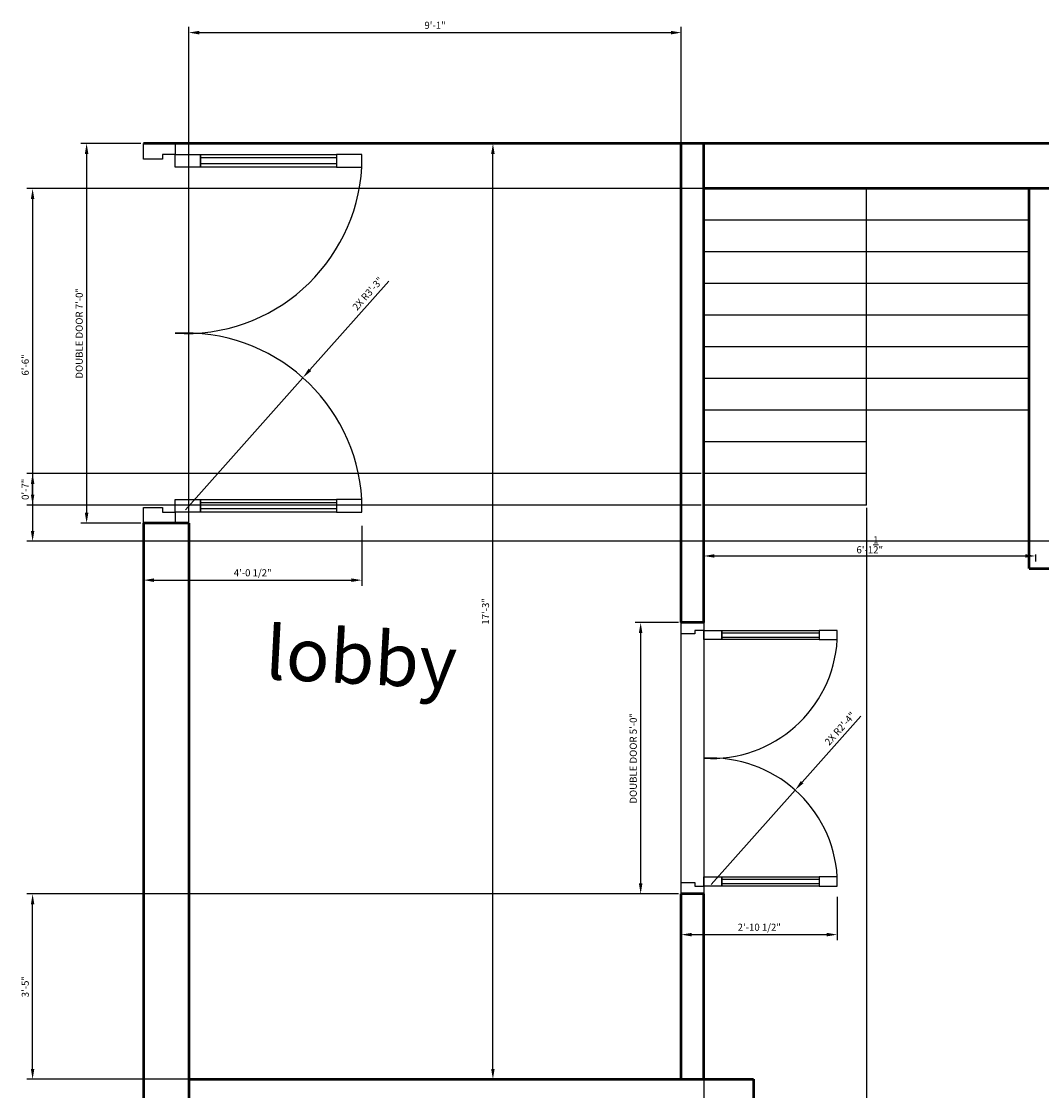
# Model space of a CAD drawing. Units: inches. Extents: x -28 to 484, y -33 to 391.
# Tile 2 of 4: x -27 to 199, y 133 to 369. Entities that reach past the tile are written whole.
import ezdxf

# ---------------------------------------------------------------- set-up
doc = ezdxf.new("R2010")
doc.units = ezdxf.units.IN
for name, color, linetype, lineweight in [('A-ANNO-DIMS', 2, 'Continuous', 18), ('A-AREA-IDEN', 7, 'Continuous', 25), ('A-DOOR', 3, 'Continuous', 25), ('A-FLOR-STRS', 7, 'Continuous', 25), ('A-WALL', 7, 'Continuous', 50)]:
    doc.layers.add(name, color=color, linetype=linetype, lineweight=lineweight)
doc.styles.get("Standard").update_dxf_attribs({"font": 'arial.ttf'})
doc.dimstyles.new('ISO-25', dxfattribs={"dimtxt": 1.5625, "dimasz": 2.3125, "dimexe": 1.25, "dimexo": 0.625, "dimtad": 1, "dimlunit": 4, "dimtxsty": 'Standard', "dimcen": 2.5, "dimadec": 0, "dimazin": 0, "dimtfac": 1, "dimtmove": 0, "dimatfit": 3, "dimfxl": 1, "dimarcsym": 0})

# ---------------------------------------------------------------- blocks, each defined once
blk = doc.blocks.new('A$C09A905BE')
for p, q in [((35, 690), (35, 610)), ((75, 690), (35, 690)), ((75, 610), (75, 690)), ((1125, 690), (1125, 610)), ((1165, 690), (1125, 690)), ((1165, 610), (1165, 690)), ((35, 610), (75, 610)), ((35, 180), (35, 610)), ((35, 610), (75, 610)), ((45, 180), (45, 610)), ((45, 610), (65, 610)), ((65, 610), (65, 180)), ((75, 610), (75, 180)), ((1125, 610), (1165, 610)), ((1125, 180), (1125, 610)), ((1125, 610), (1165, 610)), ((1135, 180), (1135, 610)), ((1135, 610), (1155, 610)), ((1155, 610), (1155, 180)), ((1165, 610), (1165, 180)), ((35, 100), (35, 180)), ((35, 180), (75, 180)), ((75, 180), (35, 180)), ((65, 180), (45, 180)), ((75, 180), (75, 100)), ((1125, 100), (1125, 180)), ((1125, 180), (1165, 180)), ((1165, 180), (1125, 180)), ((1155, 180), (1135, 180)), ((1165, 180), (1165, 100)), ((0, 0), (0, 100)), ((0, 100), (35, 100)), ((35, 100), (35, 60)), ((75, 100), (35, 100)), ((1165, 100), (1125, 100)), ((1165, 100), (1200, 100)), ((1165, 60), (1165, 100)), ((1200, 100), (1200, 0)), ((35, 60), (50, 60)), ((50, 60), (50, 50)), ((50, 50), (50, 0)), ((1150, 50), (1150, 60)), ((1150, 60), (1165, 60)), ((1150, 0), (1150, 50)), ((50, 0), (0, 0)), ((1200, 0), (1150, 0))]:
    blk.add_line(p, q)
for centre, start, end in [((42.5, 132.5), 356.6637, 86.6637), ((1157.5, 132.5), 93.3363, 183.3363)]:
    blk.add_arc(centre, 558.4, start, end)
blk = doc.blocks.new('*D13')
at = {"layer": 'A-ANNO-DIMS', "color": 0, "lineweight": -2, "transparency": 16777216}
for p, q in [((73.12, 342), (78.56, 342)), ((77.31, 137.31), (77.31, 339.69)), ((73.12, 135), (78.56, 135))]:
    blk.add_line(p, q, dxfattribs=at)
at = {"layer": 'A-ANNO-DIMS', "color": 0, "transparency": 16777216}
for points in [[(76.92, 339.69), (77.69, 339.69), (77.31, 342)], [(76.92, 137.31), (77.69, 137.31), (77.31, 135)]]:
    blk.add_solid(points, dxfattribs=at)
at = {"layer": 'Defpoints', "color": 0, "transparency": 16777216}
for p in [(72.5, 342), (77.31, 342), (72.5, 135)]:
    blk.add_point(p, dxfattribs=at)
at = {"layer": 'A-ANNO-DIMS', "color": 0, "transparency": 16777216, "insert": (75.88, 238.5), "char_height": 1.562, "attachment_point": 5, "rotation": 90}
blk.add_mtext('17\'-3"', dxfattribs=at)
blk = doc.blocks.new('*D14')
at = {"layer": 'A-ANNO-DIMS', "color": 0, "lineweight": -2, "transparency": 16777216}
for p, q in [((124, 251.07), (124, 249.5)), ((126.31, 250.75), (195.09, 250.75)), ((197.4, 251.07), (197.4, 249.5))]:
    blk.add_line(p, q, dxfattribs=at)
at = {"layer": 'A-ANNO-DIMS', "color": 0, "transparency": 16777216}
for points in [[(126.31, 251.14), (126.31, 250.37), (124, 250.75)], [(195.09, 251.14), (195.09, 250.37), (197.4, 250.75)]]:
    blk.add_solid(points, dxfattribs=at)
at = {"layer": 'Defpoints', "color": 0, "transparency": 16777216}
for p in [(124, 251.69), (197.4, 251.69), (197.4, 250.75)]:
    blk.add_point(p, dxfattribs=at)
at = {"layer": 'A-ANNO-DIMS', "color": 0, "transparency": 16777216, "insert": (160.7, 253.22), "char_height": 1.5625, "attachment_point": 5}
blk.add_mtext('6\'-1{\\H1x;\\S1/2;}"', dxfattribs=at)
blk = doc.blocks.new('*D24')
at = {"layer": 'A-ANNO-DIMS', "color": 0, "lineweight": -2, "transparency": 16777216}
for p, q in [((-0.62, 342), (-13.85, 342)), ((-12.6, 339.69), (-12.6, 260.31)), ((-0.62, 258), (-13.85, 258))]:
    blk.add_line(p, q, dxfattribs=at)
at = {"layer": 'A-ANNO-DIMS', "color": 0, "transparency": 16777216}
for points in [[(-12.99, 339.69), (-12.21, 339.69), (-12.6, 342)], [(-12.99, 260.31), (-12.21, 260.31), (-12.6, 258)]]:
    blk.add_solid(points, dxfattribs=at)
at = {"layer": 'Defpoints', "color": 0, "transparency": 16777216}
for p in [(0, 342), (-12.6, 258), (0, 258)]:
    blk.add_point(p, dxfattribs=at)
at = {"layer": 'A-ANNO-DIMS', "color": 0, "transparency": 16777216, "insert": (-14.03, 300), "char_height": 1.5625, "attachment_point": 5, "rotation": 90}
blk.add_mtext('DOUBLE DOOR 7\'-0"', dxfattribs=at)
blk = doc.blocks.new('*D25')
at = {"layer": 'A-ANNO-DIMS', "color": 0, "lineweight": -2, "transparency": 16777216}
for p, q in [((0, 257.38), (0, 244.15)), ((48.3, 257.38), (48.3, 244.15)), ((2.31, 245.4), (45.99, 245.4))]:
    blk.add_line(p, q, dxfattribs=at)
at = {"layer": 'A-ANNO-DIMS', "color": 0, "transparency": 16777216}
for points in [[(2.31, 245.79), (2.31, 245.01), (0, 245.4)], [(45.99, 245.79), (45.99, 245.01), (48.3, 245.4)]]:
    blk.add_solid(points, dxfattribs=at)
at = {"layer": 'Defpoints', "color": 0, "transparency": 16777216}
for p in [(0, 258), (48.3, 258), (48.3, 245.4)]:
    blk.add_point(p, dxfattribs=at)
at = {"layer": 'A-ANNO-DIMS', "color": 0, "transparency": 16777216, "insert": (24.15, 246.83), "char_height": 1.562, "attachment_point": 5}
blk.add_mtext('4\'-0 1/2"', dxfattribs=at)
blk = doc.blocks.new('*D26')
at = {"layer": 'A-ANNO-DIMS', "color": 0, "lineweight": -2, "transparency": 16777216}
for p, q in [((118.38, 236), (108.75, 236)), ((110, 233.69), (110, 178.31)), ((118.38, 176), (108.75, 176))]:
    blk.add_line(p, q, dxfattribs=at)
at = {"layer": 'A-ANNO-DIMS', "color": 0, "transparency": 16777216}
for points in [[(109.61, 233.69), (110.39, 233.69), (110, 236)], [(109.61, 178.31), (110.39, 178.31), (110, 176)]]:
    blk.add_solid(points, dxfattribs=at)
at = {"layer": 'Defpoints', "color": 0, "transparency": 16777216}
for p in [(119, 236), (110, 176), (119, 176)]:
    blk.add_point(p, dxfattribs=at)
at = {"layer": 'A-ANNO-DIMS', "color": 0, "transparency": 16777216, "insert": (108.57, 206), "char_height": 1.5625, "attachment_point": 5, "rotation": 90}
blk.add_mtext('DOUBLE DOOR 5\'-0"', dxfattribs=at)
blk = doc.blocks.new('*D27')
at = {"layer": 'A-ANNO-DIMS', "color": 0, "lineweight": -2, "transparency": 16777216}
for p, q in [((119, 175.38), (119, 165.75)), ((153.5, 175.38), (153.5, 165.75)), ((121.31, 167), (151.19, 167))]:
    blk.add_line(p, q, dxfattribs=at)
at = {"layer": 'A-ANNO-DIMS', "color": 0, "transparency": 16777216}
for points in [[(121.31, 167.39), (121.31, 166.61), (119, 167)], [(151.19, 167.39), (151.19, 166.61), (153.5, 167)]]:
    blk.add_solid(points, dxfattribs=at)
at = {"layer": 'Defpoints', "color": 0, "transparency": 16777216}
for p in [(119, 176), (153.5, 176), (153.5, 167)]:
    blk.add_point(p, dxfattribs=at)
at = {"layer": 'A-ANNO-DIMS', "color": 0, "transparency": 16777216, "insert": (136.25, 168.43), "char_height": 1.562, "attachment_point": 5}
blk.add_mtext('2\'-10 1/2"', dxfattribs=at)
blk = doc.blocks.new('*D30')
at = {"layer": 'A-ANNO-DIMS', "color": 0, "lineweight": -2, "transparency": 16777216}
for p, q in [((10, 135.62), (10, 367.75)), ((119, 135.62), (119, 367.75)), ((12.31, 366.5), (116.69, 366.5))]:
    blk.add_line(p, q, dxfattribs=at)
at = {"layer": 'A-ANNO-DIMS', "color": 0, "transparency": 16777216}
for points in [[(12.31, 366.89), (12.31, 366.11), (10, 366.5)], [(116.69, 366.89), (116.69, 366.11), (119, 366.5)]]:
    blk.add_solid(points, dxfattribs=at)
at = {"layer": 'Defpoints', "color": 0, "transparency": 16777216}
for p in [(119, 366.5), (10, 135), (119, 135)]:
    blk.add_point(p, dxfattribs=at)
at = {"layer": 'A-ANNO-DIMS', "color": 0, "transparency": 16777216, "insert": (64.5, 367.92), "char_height": 1.562, "attachment_point": 5}
blk.add_mtext('9\'-1"', dxfattribs=at)
blk = doc.blocks.new('*D31')
at = {"layer": 'A-ANNO-DIMS', "color": 0, "lineweight": -2, "transparency": 16777216}
for p, q in [((296.38, 332), (-25.8, 332)), ((-24.55, 329.69), (-24.55, 256.31)), ((296.38, 254), (-25.8, 254))]:
    blk.add_line(p, q, dxfattribs=at)
at = {"layer": 'A-ANNO-DIMS', "color": 0, "transparency": 16777216}
for points in [[(-24.93, 329.69), (-24.16, 329.69), (-24.55, 332)], [(-24.93, 256.31), (-24.16, 256.31), (-24.55, 254)]]:
    blk.add_solid(points, dxfattribs=at)
at = {"layer": 'Defpoints', "color": 0, "transparency": 16777216}
for p in [(297, 332), (-24.55, 254), (297, 254)]:
    blk.add_point(p, dxfattribs=at)
at = {"layer": 'A-ANNO-DIMS', "color": 0, "transparency": 16777216, "insert": (-25.97, 293), "char_height": 1.562, "attachment_point": 5, "rotation": 90}
blk.add_mtext('6\'-6"', dxfattribs=at)
blk = doc.blocks.new('*D35')
at = {"layer": 'A-ANNO-DIMS', "color": 0, "lineweight": -2, "transparency": 16777216}
for p, q in [((118.38, 176), (-25.8, 176)), ((-24.55, 137.31), (-24.55, 173.69)), ((118.38, 135), (-25.8, 135))]:
    blk.add_line(p, q, dxfattribs=at)
at = {"layer": 'A-ANNO-DIMS', "color": 0, "transparency": 16777216}
for points in [[(-24.93, 173.69), (-24.16, 173.69), (-24.55, 176)], [(-24.93, 137.31), (-24.16, 137.31), (-24.55, 135)]]:
    blk.add_solid(points, dxfattribs=at)
at = {"layer": 'Defpoints', "color": 0, "transparency": 16777216}
for p in [(-24.55, 176), (119, 176), (119, 135)]:
    blk.add_point(p, dxfattribs=at)
at = {"layer": 'A-ANNO-DIMS', "color": 0, "transparency": 16777216, "insert": (-25.97, 155.5), "char_height": 1.562, "attachment_point": 5, "rotation": 90}
blk.add_mtext('3\'-5"', dxfattribs=at)
blk = doc.blocks.new('*D36')
at = {"layer": 'A-ANNO-DIMS', "color": 0, "lineweight": -2, "transparency": 16777216}
for p, q in [((124, 261.38), (124, -25.75)), ((160, 261.38), (160, -25.75)), ((126.31, -24.5), (157.69, -24.5))]:
    blk.add_line(p, q, dxfattribs=at)
at = {"layer": 'A-ANNO-DIMS', "color": 0, "transparency": 16777216}
for points in [[(126.31, -24.11), (126.31, -24.89), (124, -24.5)], [(157.69, -24.11), (157.69, -24.89), (160, -24.5)]]:
    blk.add_solid(points, dxfattribs=at)
at = {"layer": 'Defpoints', "color": 0, "transparency": 16777216}
for p in [(124, 262), (160, 262), (160, -24.5)]:
    blk.add_point(p, dxfattribs=at)
at = {"layer": 'A-ANNO-DIMS', "color": 0, "transparency": 16777216, "insert": (142, -23.08), "char_height": 1.562, "attachment_point": 5}
blk.add_mtext('3\'-0"', dxfattribs=at)
blk = doc.blocks.new('*D37')
at = {"layer": 'A-ANNO-DIMS', "color": 0, "lineweight": -2, "transparency": 16777216}
for p, q in [((123.38, 269), (-25.8, 269)), ((-24.55, 264.31), (-24.55, 266.69)), ((123.38, 262), (-25.8, 262))]:
    blk.add_line(p, q, dxfattribs=at)
at = {"layer": 'A-ANNO-DIMS', "color": 0, "transparency": 16777216}
for points in [[(-24.93, 266.69), (-24.16, 266.69), (-24.55, 269)], [(-24.93, 264.31), (-24.16, 264.31), (-24.55, 262)]]:
    blk.add_solid(points, dxfattribs=at)
at = {"layer": 'Defpoints', "color": 0, "transparency": 16777216}
for p in [(-24.55, 269), (124, 269), (124, 262)]:
    blk.add_point(p, dxfattribs=at)
at = {"layer": 'A-ANNO-DIMS', "color": 0, "transparency": 16777216, "insert": (-25.97, 265.5), "char_height": 1.562, "attachment_point": 5, "rotation": 90}
blk.add_mtext('0\'-7"', dxfattribs=at)
blk = doc.blocks.new('*D39')
at = {"layer": 'A-ANNO-DIMS', "color": 0, "lineweight": -2, "transparency": 16777216}
for p, q in [((54.27, 311.54), (36.8, 291.91)), ((9.28, 260.98), (35.26, 290.18))]:
    blk.add_line(p, q, dxfattribs=at)
at = {"layer": 'A-ANNO-DIMS', "color": 0, "transparency": 16777216}
blk.add_solid([(36.51, 292.16), (37.09, 291.65), (35.26, 290.18)], dxfattribs=at)
at = {"layer": 'Defpoints', "color": 0, "transparency": 16777216}
for p in [(35.26, 290.18), (9.28, 260.98)]:
    blk.add_point(p, dxfattribs=at)
at = {"layer": 'A-ANNO-DIMS', "color": 0, "transparency": 16777216, "insert": (49.79, 308.65), "char_height": 1.562, "attachment_point": 5, "rotation": 48.337}
blk.add_mtext('2X R3\'-3"', dxfattribs=at)
blk = doc.blocks.new('*D42')
at = {"layer": 'A-ANNO-DIMS', "color": 0, "lineweight": -2, "transparency": 16777216}
for p, q in [((158.74, 215.34), (145.72, 200.71)), ((125.62, 178.12), (144.19, 198.98))]:
    blk.add_line(p, q, dxfattribs=at)
at = {"layer": 'A-ANNO-DIMS', "color": 0, "transparency": 16777216}
blk.add_solid([(145.44, 200.97), (146.01, 200.46), (144.19, 198.98)], dxfattribs=at)
at = {"layer": 'Defpoints', "color": 0, "transparency": 16777216}
for p in [(144.19, 198.98), (125.62, 178.12)]:
    blk.add_point(p, dxfattribs=at)
at = {"layer": 'A-ANNO-DIMS', "color": 0, "transparency": 16777216, "insert": (154.27, 212.44), "char_height": 1.562, "attachment_point": 5, "rotation": 48.3361}
blk.add_mtext('2X R2\'-4"', dxfattribs=at)

msp = doc.modelspace()

# ---------------------------------------------------------------- linework, layer by layer
at = {"layer": 'A-FLOR-STRS'}
for p, q in [((160, 262), (160, 332)), ((196, 325), (124, 325)), ((196, 318), (124, 318)), ((196, 311), (124, 311)), ((196, 304), (124, 304)), ((196, 297), (124, 297)), ((196, 290), (124, 290)), ((196, 283), (124, 283)), ((160, 276), (124, 276)), ((160, 269), (124, 269)), ((160, 262), (124, 262))]:
    msp.add_line(p, q, dxfattribs=at)
at = {"layer": 'A-WALL'}
for p, q in [((119, 342), (0, 342)), ((119, 236), (119, 342)), ((124, 236), (124, 342)), ((446, 332), (124, 332)), ((196, 248), (196, 332)), ((10, 258), (0, 258)), ((10, 258), (10, 10)), ((196, 248), (201, 248)), ((124, 236), (119, 236)), ((119, 135), (119, 176)), ((124, 176), (119, 176)), ((124, 135), (124, 176)), ((10, 135), (135, 135)), ((135, 135), (135, 130))]:
    msp.add_line(p, q, dxfattribs=at)
msp.add_lwpolyline([(0, 258), (0, 0), (456, 0), (456, 342), (0, 342)], dxfattribs=at)

# ---------------------------------------------------------------- block references
at = {"layer": 'A-DOOR', "rotation": 270}
for p, xscale, yscale, zscale in [((0, 342), 0.0699999999999999, 0.0699999999999999, 0.0699999999999999), ((119, 236), 0.05, 0.05, 0.05)]:
    msp.add_blockref('A$C09A905BE', p, dxfattribs=dict(at, xscale=xscale, yscale=yscale, zscale=zscale))

# ---------------------------------------------------------------- texts
at = {"layer": 'A-AREA-IDEN'}
msp.add_text('lobby', height=11.7233, rotation=356.97653, dxfattribs=at).set_placement((26.722, 223.546))

# ---------------------------------------------------------------- dimensions: what is measured, and where the dimension line sits
at = {"layer": 'A-ANNO-DIMS'}
for base, p1, p2, override, picture, middle in [((119, 366.5), (10, 135), (119, 135), {"dimdec": 1, "dimlfac": 1, "dimrnd": 0, "dimzin": 1, "dimdsep": 46, "dimlunit": 4, "dimfrac": 2}, '*D30', (64.5, 367.923)), ((160, -24.5), (124, 262), (160, 262), {"dimdec": 1, "dimlfac": 1, "dimrnd": 0, "dimzin": 1, "dimdsep": 46, "dimlunit": 4, "dimfrac": 2}, '*D36', (142, -23.077)), ((48.3, 245.4), (0, 258), (48.3, 258), {"dimdec": 1, "dimlfac": 1, "dimrnd": 0, "dimzin": 1, "dimdsep": 46, "dimlunit": 4, "dimfrac": 2}, '*D25', (24.15, 246.833)), ((197.404, 250.752), (124, 251.693), (197.404, 251.693), {"dimclrd": 0, "dimclre": 0, "dimclrt": 0}, '*D14', (160.702, 253.219)), ((153.5, 167), (119, 176), (153.5, 176), {"dimdec": 1, "dimlfac": 1, "dimrnd": 0, "dimzin": 1, "dimdsep": 46, "dimlunit": 4, "dimfrac": 2}, '*D27', (136.25, 168.433))]:
    dim = msp.add_linear_dim(base=base, p1=p1, p2=p2, dimstyle='ISO-25', override=override, dxfattribs=at)
    dim.commit()
    dim.dimension.update_dxf_attribs({"geometry": picture, "text_midpoint": middle})
for base, p1, p2, picture, middle in [((-12.6, 258), (0, 342), (0, 258), '*D24', (-14.033, 300)), ((110, 176), (119, 236), (119, 176), '*D26', (108.567, 206))]:
    dim = msp.add_linear_dim(base=base, p1=p1, p2=p2, angle=270, text='DOUBLE DOOR <>', dimstyle='ISO-25', override={"dimdec": 1, "dimlfac": 1, "dimrnd": 0, "dimzin": 1, "dimdsep": 46, "dimlunit": 4, "dimfrac": 2}, dxfattribs=at)
    dim.commit()
    dim.dimension.update_dxf_attribs({"geometry": picture, "text_midpoint": middle})
for base, p1, p2, override, picture, middle in [((77.307, 342), (72.5, 135), (72.5, 342), {"dimclrd": 0, "dimclre": 0, "dimclrt": 0}, '*D13', (75.884, 238.5)), ((-24.546, 254), (297, 332), (297, 254), {"dimdec": 1, "dimlfac": 1, "dimrnd": 0, "dimzin": 1, "dimdsep": 46, "dimlunit": 4, "dimfrac": 2}, '*D31', (-25.969, 293)), ((-24.546, 269), (124, 262), (124, 269), {"dimdec": 1, "dimlfac": 1, "dimrnd": 0, "dimzin": 1, "dimdsep": 46, "dimlunit": 4, "dimfrac": 2}, '*D37', (-25.969, 265.5)), ((-24.546, 176), (119, 135), (119, 176), {"dimdec": 1, "dimlfac": 1, "dimrnd": 0, "dimzin": 1, "dimdsep": 46, "dimlunit": 4, "dimfrac": 2}, '*D35', (-25.969, 155.5))]:
    dim = msp.add_linear_dim(base=base, p1=p1, p2=p2, angle=90, dimstyle='ISO-25', override=override, dxfattribs=at)
    dim.commit()
    dim.dimension.update_dxf_attribs({"geometry": picture, "text_midpoint": middle})
for center, mpoint, picture, middle in [((9.275, 260.975), (35.261, 290.179), '*D39', (50.852, 307.701)), ((125.625, 178.125), (144.187, 198.985), '*D42', (155.324, 211.5))]:
    dim = msp.add_radius_dim(center=center, mpoint=mpoint, text='2X <>', dimstyle='ISO-25', override={"dimdec": 1, "dimlfac": 1, "dimrnd": 0, "dimzin": 1, "dimdsep": 46, "dimlunit": 4, "dimfrac": 2}, dxfattribs=at)
    dim.commit()
    dim.dimension.update_dxf_attribs({"geometry": picture, "text_midpoint": middle, "dimtype": 164})

doc.saveas('drawing.dxf')
